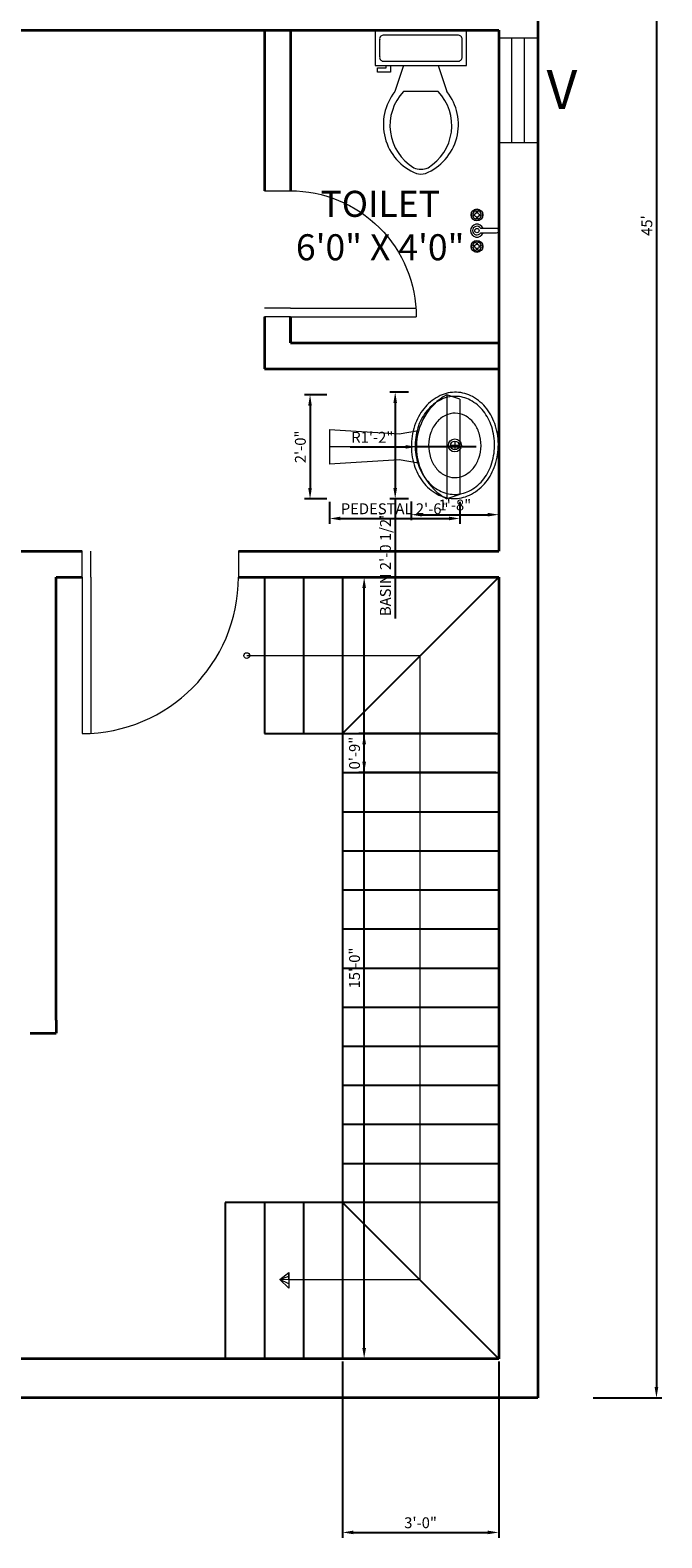
# Model space of a CAD drawing. Units: inches. Extents: x 2009 to 2890, y 2827 to 3504.
# Tile 5 of 6: x 2741 to 2886, y 2867 to 3214. Entities that reach past the tile are written whole.
import ezdxf

# ---------------------------------------------------------------- set-up
doc = ezdxf.new("R2010")
doc.units = ezdxf.units.IN
for name, color, linetype, lineweight in [('A-ANNO-DIMS', 2, 'Continuous', 18), ('A-ANNO-SYMB', 2, 'Continuous', 18), ('A-ANNO-TEXT', 3, 'Continuous', 18), ('A-AREA-IDEN', 7, 'Continuous', 25), ('A-DOOR', 3, 'Continuous', 18), ('A-FLOR-FIXT', 9, 'Continuous', 18), ('A-FLOR-STRS', 7, 'Continuous', 25), ('A-GLAZ', 4, 'Continuous', 18), ('A-WALL', 7, 'Continuous', 35)]:
    doc.layers.add(name, color=color, linetype=linetype, lineweight=lineweight)
doc.styles.get("Standard").update_dxf_attribs({"font": 'arial.ttf'})
doc.dimstyles.new('ISO-25', dxfattribs={"dimtxt": 2.5, "dimasz": 2.5, "dimexe": 1.25, "dimexo": 0.625, "dimtad": 1, "dimdec": 0, "dimlunit": 3, "dimtxsty": 'Standard', "dimcen": 2.5, "dimadec": 0, "dimazin": 0, "dimtfac": 1, "dimtdec": 0, "dimtmove": 0, "dimatfit": 3, "dimfxl": 1, "dimarcsym": 0})

# ---------------------------------------------------------------- blocks, each defined once
blk = doc.blocks.new('*D14')
at = {"layer": 'A-ANNO-DIMS', "color": 0, "lineweight": -2, "transparency": 16777216}
for p, q in [((2858.24, 3438.94), (2886.22, 3438.94)), ((2884.97, 3436.44), (2884.97, 2901.44)), ((2870.41, 2898.94), (2886.22, 2898.94))]:
    blk.add_line(p, q, dxfattribs=at)
at = {"layer": 'A-ANNO-DIMS', "color": 0, "transparency": 16777216}
for points in [[(2884.55, 3436.44), (2885.39, 3436.44), (2884.97, 3438.94)], [(2884.55, 2901.44), (2885.39, 2901.44), (2884.97, 2898.94)]]:
    blk.add_solid(points, dxfattribs=at)
at = {"layer": 'Defpoints', "color": 0, "transparency": 16777216}
for p in [(2857.61, 3438.94), (2869.79, 2898.94), (2884.97, 2898.94)]:
    blk.add_point(p, dxfattribs=at)
at = {"layer": 'A-ANNO-DIMS', "color": 0, "transparency": 16777216, "insert": (2883.07, 3168.94), "char_height": 2.5, "attachment_point": 5, "rotation": 90}
blk.add_mtext("45'", dxfattribs=at)
blk = doc.blocks.new('Toilet - top')
for p, q in [((9.5, -6), (9.5, -2)), ((-10, -8.5), (-8, -8.5)), ((-10, -9.5), (-10, -8.5)), ((-7, -9.5), (-10, -9.5)), ((-8, -8.5), (-8, -8)), ((-7, -8), (-7, -9.5)), ((-4, -8), (-6, -14)), ((4, -8), (6, -14)), ((4, -14), (-4, -14))]:
    blk.add_line(p, q)
blk.add_lwpolyline([(10.5, -8), (10.5, 0), (-10.5, 0), (-10.5, -8)], close=True)
for points in [[(-9.5, -2), (-9.5, -6)], [(8.5, -1), (-8.5, -1)], [(-8.5, -7), (8.5, -7)]]:
    blk.add_lwpolyline(points)
for centre, radius, start, end in [((-8.62, -1.88), 0.884, 81.8699, 188.1301), ((8.62, -1.88), 0.884, 351.8699, 98.1301), ((-8.62, -6.12), 0.884, 171.8699, 278.1301), ((8.62, -6.12), 0.884, 261.8699, 8.1301), ((3.52, -21.58), 12.17, 141.4691, 247.9714), ((4.2, -21.82), 11.33, 136.3677, 238.9468), ((-3.52, -21.58), 12.17, 292.0284, 38.5307), ((-4.2, -21.82), 11.33, 301.053, 43.6321), ((0, -27.88), 4, 245.7318, 294.2682), ((0, -29), 4, 254.8605, 285.1395)]:
    blk.add_arc(centre, radius, start, end)
blk = doc.blocks.new('Faucet - Bathroom top')
for p, q in [((-4.107, 0.125), (-4.375, 0.125)), ((-3.75, 0.4788), (-3.75, 0.75)), ((-3.5, 0.482), (-3.5, 0.75)), ((-3.1461, 0.125), (-2.875, 0.125)), ((3.143, 0.125), (2.875, 0.125)), ((3.5, 0.4788), (3.5, 0.75)), ((3.75, 0.482), (3.75, 0.75)), ((4.1039, 0.125), (4.375, 0.125)), ((-4.1039, -0.125), (-4.375, -0.125)), ((-3.75, -0.4821), (-3.75, -0.75)), ((-3.5, -0.4789), (-3.5, -0.75)), ((-3.143, -0.125), (-2.875, -0.125)), ((-0.5, -0.8639), (-0.5, -4.5)), ((0.5, -4.5), (0.5, -0.8631)), ((3.1461, -0.125), (2.875, -0.125)), ((3.5, -0.4821), (3.5, -0.75)), ((3.75, -0.4789), (3.75, -0.75)), ((4.107, -0.125), (4.375, -0.125))]:
    blk.add_line(p, q)
for centre, radius in [((-3.625, 0), 1.375), ((-4.625, 0), 0.2795), ((-3.625, 0), 0.5), ((-3.625, 1), 0.2795), ((-2.625, 0), 0.2795), ((0, 0), 0.5), ((3.625, 0), 1.375), ((2.625, 0), 0.2795), ((3.625, 0), 0.5), ((3.625, 1), 0.2795), ((4.625, 0), 0.2795), ((-3.625, -1), 0.2795), ((3.625, -1), 0.2795)]:
    blk.add_circle(centre, radius)
for centre, radius, start, end in [((-3.625, 0), 1, 105.2407, 164.2093), ((-3.625, 0), 1, 16.44125, 74.07887), ((0, 0), 1.5, 289.6514, 250.3603), ((0, 0), 1, 300.3431, 239.7554), ((3.625, 0), 1, 106.12, 164.0884), ((3.625, 0), 1, 16.23422, 73.90469), ((-3.625, 0), 1, 196.2342, 253.9047), ((-3.625, 0), 1, 286.12, 344.0884), ((3.625, 0), 1, 196.4413, 254.0789), ((3.625, 0), 1, 285.2407, 344.2093), ((0, -4.5), 0.5, 180, 0)]:
    blk.add_arc(centre, radius, start, end)
blk = doc.blocks.new('Sink - Oval top')
for p, q in [((-1, 0), (1, 0)), ((0, 1), (0, -1))]:
    blk.add_line(p, q)
for points in [[(-12.23, 0.39, 0.117634), (-11.46, -3.36, 0.104469), (-8.88, -6.8, 0.090016), (-5.08, -9.07, 0.08192), (-0.32, -10.02, 0.08192), (4.49, -9.38, 0.090016), (8.42, -7.36, 0.104469), (11.22, -4.09, 0.117634), (12.23, -0.39, 0.117634), (11.46, 3.36, 0.104469), (8.88, 6.8, 0.090016), (5.08, 9.07, 0.08192), (0.32, 10.02, 0.08192), (-4.49, 9.38, 0.090016), (-8.42, 7.36, 0.104469), (-11.22, 4.09, 0.117634)], [(-11.29, 0.16, 0.118622), (-10.52, -3.25, 0.104678), (-8.07, -6.36, 0.089562), (-4.54, -8.37, 0.081185), (-0.13, -9.15, 0.081185), (4.3, -8.49, 0.089562), (7.89, -6.58, 0.104678), (10.42, -3.55, 0.118622), (11.29, -0.16, 0.118622), (10.52, 3.25, 0.104678), (8.07, 6.36, 0.089562), (4.54, 8.37, 0.081185), (0.13, 9.15, 0.081185), (-4.3, 8.49, 0.089562), (-7.89, 6.58, 0.104678), (-10.42, 3.55, 0.118622)], [(-7.42, 0.08, 0.118283), (-6.91, -2.17, 0.104607), (-5.29, -4.21, 0.089718), (-2.97, -5.53, 0.081436), (-0.07, -6.04, 0.081436), (2.84, -5.59, 0.089718), (5.2, -4.33, 0.104607), (6.86, -2.32, 0.118283), (7.42, -0.08, 0.118283), (6.91, 2.17, 0.104607), (5.29, 4.21, 0.089718), (2.97, 5.53, 0.081436), (0.07, 6.04, 0.081436), (-2.84, 5.59, 0.089718), (-5.2, 4.33, 0.104607), (-6.86, 2.32, 0.118283)]]:
    blk.add_lwpolyline(points, format="xyb", close=True)
for radius in [1.5, 1]:
    blk.add_circle((0, 0), radius)
blk = doc.blocks.new('Sink - Pedestal elevation')
for p, q in [((-11, 30), (-12, 27)), ((-11, 30), (11, 30)), ((11, 30), (12, 27)), ((-12, 27), (12, 27)), ((-3, 16), (-3.7523, 20.5139)), ((0, 20), (0, 0)), ((3.7527, 20.5157), (3, 16)), ((-4, 0), (-3, 16)), ((3, 16), (4, 0)), ((-4, 0), (4, 0))]:
    blk.add_line(p, q)
blk.add_arc((0, 33.7857), 13.7857, 209.4871, 330.5129)
blk = doc.blocks.new('VENT-24IN')
for p, q in [((0, 24), (0, 0)), ((9, 24), (0, 24)), ((3, 24), (3, 0)), ((6, 0), (6, 24)), ((9, 0), (9, 24)), ((0, 0), (9, 0))]:
    blk.add_line(p, q)
blk = doc.blocks.new('DOOR-29IN')
for p, q in [((0, 35), (0, 29)), ((27, 29), (27, 35)), ((29, 29), (29, 35)), ((27, 29), (27, 0)), ((29, 29), (29, 0))]:
    blk.add_line(p, q)
blk.add_arc((29, 29), 29, 180, 270)
blk = doc.blocks.new('DOOR-36IN')
for p, q in [((34, 6), (34, 42)), ((36, 6), (36, 42)), ((0, 0), (0, 6)), ((34, 6), (34, 0)), ((36, 6), (36, 0))]:
    blk.add_line(p, q)
blk.add_arc((36, 6), 36, 90, 180)
blk = doc.blocks.new('*D61')
at = {"layer": 'A-ANNO-DIMS', "color": 0, "lineweight": -2, "transparency": 16777216}
for p, q in [((2827.82, 3130.58), (2823.51, 3130.58)), ((2824.76, 3128.08), (2824.76, 3108.53)), ((2827.82, 3106.03), (2823.51, 3106.03)), ((2824.76, 3106.03), (2824.76, 3078.47))]:
    blk.add_line(p, q, dxfattribs=at)
at = {"layer": 'A-ANNO-DIMS', "color": 0, "transparency": 16777216}
for points in [[(2824.34, 3128.08), (2825.18, 3128.08), (2824.76, 3130.58)], [(2824.34, 3108.53), (2825.18, 3108.53), (2824.76, 3106.03)]]:
    blk.add_solid(points, dxfattribs=at)
at = {"layer": 'Defpoints', "color": 0, "transparency": 16777216}
for p in [(2828.44, 3130.58), (2824.76, 3106.03), (2828.44, 3106.03)]:
    blk.add_point(p, dxfattribs=at)
at = {"layer": 'A-ANNO-DIMS', "color": 0, "transparency": 16777216, "insert": (2822.84, 3091), "char_height": 2.5, "attachment_point": 5, "rotation": 90}
blk.add_mtext('BASIN 2\'-0 1/2"', dxfattribs=at)
blk = doc.blocks.new('*D62')
at = {"layer": 'A-ANNO-DIMS', "color": 0, "lineweight": -2, "transparency": 16777216}
for p, q in [((2828.44, 3105.41), (2828.44, 3101.1)), ((2848.58, 3105.41), (2848.58, 3101.1)), ((2830.94, 3102.35), (2846.08, 3102.35))]:
    blk.add_line(p, q, dxfattribs=at)
at = {"layer": 'A-ANNO-DIMS', "color": 0, "transparency": 16777216}
for points in [[(2830.94, 3102.77), (2830.94, 3101.93), (2828.44, 3102.35)], [(2846.08, 3102.77), (2846.08, 3101.93), (2848.58, 3102.35)]]:
    blk.add_solid(points, dxfattribs=at)
at = {"layer": 'Defpoints', "color": 0, "transparency": 16777216}
for p in [(2828.44, 3106.03), (2848.58, 3106.03), (2848.58, 3102.35)]:
    blk.add_point(p, dxfattribs=at)
at = {"layer": 'A-ANNO-DIMS', "color": 0, "transparency": 16777216, "insert": (2838.51, 3104.25), "char_height": 2.5, "attachment_point": 5}
blk.add_mtext('1\'-8"', dxfattribs=at)
blk = doc.blocks.new('*D63')
at = {"layer": 'A-ANNO-DIMS', "color": 0, "lineweight": -2, "transparency": 16777216}
for p, q in [((2809.64, 3105.34), (2809.64, 3100.22)), ((2839.64, 3105.34), (2839.64, 3100.22)), ((2812.14, 3101.47), (2837.14, 3101.47))]:
    blk.add_line(p, q, dxfattribs=at)
at = {"layer": 'A-ANNO-DIMS', "color": 0, "transparency": 16777216}
for points in [[(2812.14, 3101.89), (2812.14, 3101.05), (2809.64, 3101.47)], [(2837.14, 3101.89), (2837.14, 3101.05), (2839.64, 3101.47)]]:
    blk.add_solid(points, dxfattribs=at)
at = {"layer": 'Defpoints', "color": 0, "transparency": 16777216}
for p in [(2809.64, 3105.97), (2839.64, 3105.97), (2839.64, 3101.47)]:
    blk.add_point(p, dxfattribs=at)
at = {"layer": 'A-ANNO-DIMS', "color": 0, "transparency": 16777216, "insert": (2824.64, 3103.39), "char_height": 2.5, "attachment_point": 5}
blk.add_mtext('PEDESTAL 2\'-6"', dxfattribs=at)
blk = doc.blocks.new('*D64')
at = {"layer": 'A-ANNO-DIMS', "color": 0, "lineweight": -2, "transparency": 16777216}
for p, q in [((2809.01, 3129.97), (2803.89, 3129.97)), ((2805.14, 3127.47), (2805.14, 3108.47)), ((2809.01, 3105.97), (2803.89, 3105.97))]:
    blk.add_line(p, q, dxfattribs=at)
at = {"layer": 'A-ANNO-DIMS', "color": 0, "transparency": 16777216}
for points in [[(2804.72, 3127.47), (2805.55, 3127.47), (2805.14, 3129.97)], [(2804.72, 3108.47), (2805.55, 3108.47), (2805.14, 3105.97)]]:
    blk.add_solid(points, dxfattribs=at)
at = {"layer": 'Defpoints', "color": 0, "transparency": 16777216}
for p in [(2809.64, 3129.97), (2805.14, 3105.97), (2809.64, 3105.97)]:
    blk.add_point(p, dxfattribs=at)
at = {"layer": 'A-ANNO-DIMS', "color": 0, "transparency": 16777216, "insert": (2803.23, 3117.97), "char_height": 2.5, "attachment_point": 5, "rotation": 90}
blk.add_mtext('2\'-0"', dxfattribs=at)
blk = doc.blocks.new('*D72')
at = {"layer": 'A-ANNO-DIMS', "color": 0, "lineweight": -2, "transparency": 16777216}
for p, q in [((2812.61, 2907.32), (2812.61, 2866.69)), ((2848.61, 2907.32), (2848.61, 2866.69)), ((2815.11, 2867.94), (2846.11, 2867.94))]:
    blk.add_line(p, q, dxfattribs=at)
at = {"layer": 'A-ANNO-DIMS', "color": 0, "transparency": 16777216}
for points in [[(2815.11, 2868.36), (2815.11, 2867.53), (2812.61, 2867.94)], [(2846.11, 2868.36), (2846.11, 2867.53), (2848.61, 2867.94)]]:
    blk.add_solid(points, dxfattribs=at)
at = {"layer": 'Defpoints', "color": 0, "transparency": 16777216}
for p in [(2812.61, 2907.94), (2848.61, 2907.94), (2848.61, 2867.94)]:
    blk.add_point(p, dxfattribs=at)
at = {"layer": 'A-ANNO-DIMS', "color": 0, "transparency": 16777216, "insert": (2830.61, 2869.85), "char_height": 2.5, "attachment_point": 5}
blk.add_mtext('3\'-0"', dxfattribs=at)
blk = doc.blocks.new('*D73')
at = {"layer": 'A-ANNO-DIMS', "color": 0, "lineweight": -2, "transparency": 16777216}
for p, q in [((2847.99, 3087.94), (2816.36, 3087.94)), ((2817.61, 2910.44), (2817.61, 3085.44)), ((2847.99, 2907.94), (2816.36, 2907.94))]:
    blk.add_line(p, q, dxfattribs=at)
at = {"layer": 'A-ANNO-DIMS', "color": 0, "transparency": 16777216}
for points in [[(2817.19, 3085.44), (2818.03, 3085.44), (2817.61, 3087.94)], [(2817.19, 2910.44), (2818.03, 2910.44), (2817.61, 2907.94)]]:
    blk.add_solid(points, dxfattribs=at)
at = {"layer": 'Defpoints', "color": 0, "transparency": 16777216}
for p in [(2817.61, 3087.94), (2848.61, 3087.94), (2848.61, 2907.94)]:
    blk.add_point(p, dxfattribs=at)
at = {"layer": 'A-ANNO-DIMS', "color": 0, "transparency": 16777216, "insert": (2815.71, 2997.94), "char_height": 2.5, "attachment_point": 5, "rotation": 90}
blk.add_mtext('15\'-0"', dxfattribs=at)
blk = doc.blocks.new('*D80')
at = {"layer": 'A-ANNO-DIMS', "color": 0, "lineweight": -2, "transparency": 16777216}
for p, q in [((2847.99, 3051.94), (2816.36, 3051.94)), ((2817.61, 3045.44), (2817.61, 3049.44)), ((2847.99, 3042.94), (2816.36, 3042.94))]:
    blk.add_line(p, q, dxfattribs=at)
at = {"layer": 'A-ANNO-DIMS', "color": 0, "transparency": 16777216}
for points in [[(2817.19, 3049.44), (2818.03, 3049.44), (2817.61, 3051.94)], [(2817.19, 3045.44), (2818.03, 3045.44), (2817.61, 3042.94)]]:
    blk.add_solid(points, dxfattribs=at)
at = {"layer": 'Defpoints', "color": 0, "transparency": 16777216}
for p in [(2817.61, 3051.94), (2848.61, 3051.94), (2848.61, 3042.94)]:
    blk.add_point(p, dxfattribs=at)
at = {"layer": 'A-ANNO-DIMS', "color": 0, "transparency": 16777216, "insert": (2815.71, 3047.44), "char_height": 2.5, "attachment_point": 5, "rotation": 90}
blk.add_mtext('0\'-9"', dxfattribs=at)
blk = doc.blocks.new('*D90')
at = {"layer": 'A-ANNO-DIMS', "color": 0, "lineweight": -2, "transparency": 16777216}
for p, q in [((2814.35, 3117.97), (2827.14, 3117.97)), ((2843.42, 3117.97), (2829.64, 3117.97))]:
    blk.add_line(p, q, dxfattribs=at)
at = {"layer": 'A-ANNO-DIMS', "color": 0, "transparency": 16777216}
blk.add_solid([(2827.14, 3118.39), (2827.14, 3117.55), (2829.64, 3117.97)], dxfattribs=at)
at = {"layer": 'Defpoints', "color": 0, "transparency": 16777216}
for p in [(2829.64, 3117.97), (2843.42, 3117.97)]:
    blk.add_point(p, dxfattribs=at)
at = {"layer": 'A-ANNO-DIMS', "color": 0, "transparency": 16777216, "insert": (2819.49, 3119.85), "char_height": 2.5, "attachment_point": 5, "rotation": 359.9983}
blk.add_mtext('R1\'-2"', dxfattribs=at)

msp = doc.modelspace()

# ---------------------------------------------------------------- linework, layer by layer
at = {"layer": 'A-ANNO-SYMB'}
for p, q in [((2790.55, 3069.9), (2830.45, 3069.9)), ((2830.45, 3069.9), (2830.45, 2926.12)), ((2798.14, 2926.16), (2800.23, 2927.83)), ((2800.23, 2926.12), (2800.23, 2927.83)), ((2800.23, 2927.83), (2800.23, 2924.18)), ((2800.23, 2927.83), (2800.23, 2926.12)), ((2798.14, 2926.16), (2800.23, 2926.98)), ((2800.23, 2924.18), (2798.14, 2926.16)), ((2800.23, 2926.12), (2798.14, 2926.16)), ((2800.23, 2925.17), (2798.14, 2926.16)), ((2800.23, 2926.98), (2800.23, 2925.17)), ((2830.45, 2926.12), (2800.23, 2926.12))]:
    msp.add_line(p, q, dxfattribs=at)
msp.add_circle((2790.55, 3069.9), 0.653, dxfattribs=at)
at = {"layer": 'A-FLOR-STRS'}
for p, q in [((2794.61, 3087.94), (2794.61, 3051.94)), ((2803.61, 3087.94), (2803.61, 3051.94)), ((2812.61, 3087.94), (2812.61, 2907.94)), ((2812.61, 3051.94), (2848.61, 3087.94)), ((2794.61, 3051.94), (2848.61, 3051.94)), ((2812.61, 3042.94), (2848.61, 3042.94)), ((2812.61, 3033.94), (2848.61, 3033.94)), ((2812.61, 3024.94), (2848.61, 3024.94)), ((2812.61, 3015.94), (2848.61, 3015.94)), ((2812.61, 3006.94), (2848.61, 3006.94)), ((2812.61, 2997.94), (2848.61, 2997.94)), ((2812.61, 2988.94), (2848.61, 2988.94)), ((2812.61, 2979.94), (2848.61, 2979.94)), ((2812.61, 2970.94), (2848.61, 2970.94)), ((2812.61, 2961.94), (2848.61, 2961.94)), ((2812.61, 2952.94), (2848.61, 2952.94)), ((2848.61, 2943.94), (2785.61, 2943.94)), ((2785.61, 2943.94), (2785.61, 2907.94)), ((2794.61, 2943.94), (2794.61, 2907.94)), ((2803.61, 2943.94), (2803.61, 2907.94)), ((2848.61, 2907.94), (2812.61, 2943.94))]:
    msp.add_line(p, q, dxfattribs=at)
at = {"layer": 'A-WALL'}
for p, q in [((2857.61, 3438.94), (2857.61, 2898.94)), ((2710.61, 3213.94), (2848.61, 3213.94)), ((2794.61, 3213.94), (2794.61, 3176.94)), ((2800.61, 3213.94), (2800.61, 3176.94)), ((2848.61, 3213.94), (2848.61, 3093.94)), ((2794.61, 3147.94), (2794.61, 3135.94)), ((2800.61, 3141.94), (2800.61, 3147.94)), ((2800.61, 3147.94), (2800.61, 3141.94)), ((2800.61, 3141.94), (2848.61, 3141.94)), ((2794.61, 3135.94), (2848.61, 3135.94)), ((2674.61, 3093.94), (2752.61, 3093.94)), ((2788.61, 3093.94), (2848.61, 3093.94)), ((2746.61, 2985.94), (2746.61, 3087.94)), ((2746.61, 3087.94), (2752.61, 3087.94)), ((2746.61, 3087.94), (2746.61, 3087.94)), ((2746.61, 3087.94), (2752.61, 3087.94)), ((2788.61, 3087.94), (2848.61, 3087.94)), ((2848.61, 3087.94), (2848.61, 2907.94)), ((2740.61, 2982.94), (2746.61, 2982.94)), ((2746.61, 2985.94), (2746.61, 2982.94)), ((2848.61, 2907.94), (2506.61, 2907.94)), ((2857.61, 2898.94), (2497.61, 2898.94))]:
    msp.add_line(p, q, dxfattribs=at)

# ---------------------------------------------------------------- block references
at = {"layer": 'A-DOOR', "extrusion": (0, 0, -1), "zscale": -1, "rotation": 269.9999999999987}
msp.add_blockref('DOOR-29IN', (-2829.61, 3176.94), dxfattribs=at)
at = {"layer": 'A-DOOR', "rotation": 180}
msp.add_blockref('DOOR-36IN', (2788.61, 3093.94), dxfattribs=at)
at = {"layer": 'A-FLOR-FIXT'}
msp.add_blockref('Toilet - top', (2830.68, 3213.79), dxfattribs=at)
for name, p, rotation in [('Faucet - Bathroom top', (2843.61, 3167.77), 90), ('Sink - Pedestal elevation', (2809.64, 3117.97), 270), ('Sink - Oval top', (2838.51, 3118.31), 270)]:
    msp.add_blockref(name, p, dxfattribs=dict(at, rotation=rotation))
at = {"layer": 'A-GLAZ', "rotation": 180}
msp.add_blockref('VENT-24IN', (2857.57, 3212.1), dxfattribs=at)

# ---------------------------------------------------------------- texts
at = {"layer": 'A-ANNO-TEXT', "insert": (2834.3, 3204.75), "char_height": 9, "attachment_point": 1}
msp.add_mtext_dynamic_manual_height_columns('\\pxqc;V', width=57.7621, gutter_width=12.5, heights=[0], dxfattribs=at)
at = {"layer": 'A-AREA-IDEN', "insert": (2794.61, 3176.94), "char_height": 6, "attachment_point": 1}
msp.add_mtext_dynamic_manual_height_columns('\\pxqc;TOILET\\P6\'0" X 4\'0" ', width=53.3807, gutter_width=12.5, heights=[0], dxfattribs=at)

# ---------------------------------------------------------------- dimensions: what is measured, and where the dimension line sits
at = {"layer": 'A-ANNO-DIMS'}
for base, p1, p2, angle, override, picture, middle in [((2884.97, 2898.94), (2857.61, 3438.94), (2869.79, 2898.94), 90, {"dimclrd": 0, "dimclre": 0, "dimclrt": 0}, '*D14', (2883.07, 3168.94)), ((2805.14, 3105.97), (2809.64, 3129.97), (2809.64, 3105.97), 270, {"dimdec": 1, "dimlfac": 1, "dimrnd": 0, "dimzin": 1, "dimdsep": 46, "dimlunit": 4, "dimfrac": 2}, '*D64', (2803.23, 3117.97)), ((2817.61, 3087.94), (2848.61, 2907.94), (2848.61, 3087.94), 90, {"dimdec": 1, "dimlfac": 1, "dimrnd": 0, "dimzin": 1, "dimdsep": 46, "dimlunit": 4, "dimfrac": 2}, '*D73', (2815.71, 2997.94)), ((2817.61, 3051.94), (2848.61, 3042.94), (2848.61, 3051.94), 90, {"dimdec": 1, "dimlfac": 1, "dimrnd": 0, "dimzin": 1, "dimdsep": 46, "dimlunit": 4, "dimfrac": 2}, '*D80', (2815.71, 3047.44))]:
    dim = msp.add_linear_dim(base=base, p1=p1, p2=p2, angle=angle, dimstyle='ISO-25', override=override, dxfattribs=at)
    dim.commit()
    dim.dimension.update_dxf_attribs({"geometry": picture, "text_midpoint": middle})
dim = msp.add_linear_dim(base=(2824.7603, 3106.0331), p1=(2828.4429, 3130.584), p2=(2828.4429, 3106.0331), angle=270, text='BASIN <>', dimstyle='ISO-25', override={"dimdec": 1, "dimlfac": 1, "dimrnd": 0, "dimzin": 1, "dimdsep": 46, "dimlunit": 4, "dimfrac": 2}, dxfattribs=at)
dim.commit()
dim.dimension.update_dxf_attribs({"geometry": '*D61', "text_midpoint": (2822.8427, 3091.0024)})
dim = msp.add_radius_dim(center=(2843.42, 3117.97), mpoint=(2829.64, 3117.97), dimstyle='ISO-25', override={"dimdec": 1, "dimlfac": 1, "dimrnd": 0, "dimzin": 1, "dimdsep": 46, "dimlunit": 4, "dimfrac": 2}, dxfattribs=at)
dim.commit()
dim.dimension.update_dxf_attribs({"geometry": '*D90', "text_midpoint": (2819.49, 3119.85)})
dim = msp.add_linear_dim(base=(2839.64, 3101.47), p1=(2809.64, 3105.97), p2=(2839.64, 3105.97), text='PEDESTAL <>', dimstyle='ISO-25', override={"dimdec": 1, "dimlfac": 1, "dimrnd": 0, "dimzin": 1, "dimdsep": 46, "dimlunit": 4, "dimfrac": 2}, dxfattribs=at)
dim.commit()
dim.dimension.update_dxf_attribs({"geometry": '*D63', "text_midpoint": (2824.64, 3103.39)})
for base, p1, p2, picture, middle in [((2848.58, 3102.35), (2828.44, 3106.03), (2848.58, 3106.03), '*D62', (2838.51, 3104.25)), ((2848.61, 2867.94), (2812.61, 2907.94), (2848.61, 2907.94), '*D72', (2830.61, 2869.85))]:
    dim = msp.add_linear_dim(base=base, p1=p1, p2=p2, dimstyle='ISO-25', override={"dimdec": 1, "dimlfac": 1, "dimrnd": 0, "dimzin": 1, "dimdsep": 46, "dimlunit": 4, "dimfrac": 2}, dxfattribs=at)
    dim.commit()
    dim.dimension.update_dxf_attribs({"geometry": picture, "text_midpoint": middle})

doc.saveas('drawing.dxf')
